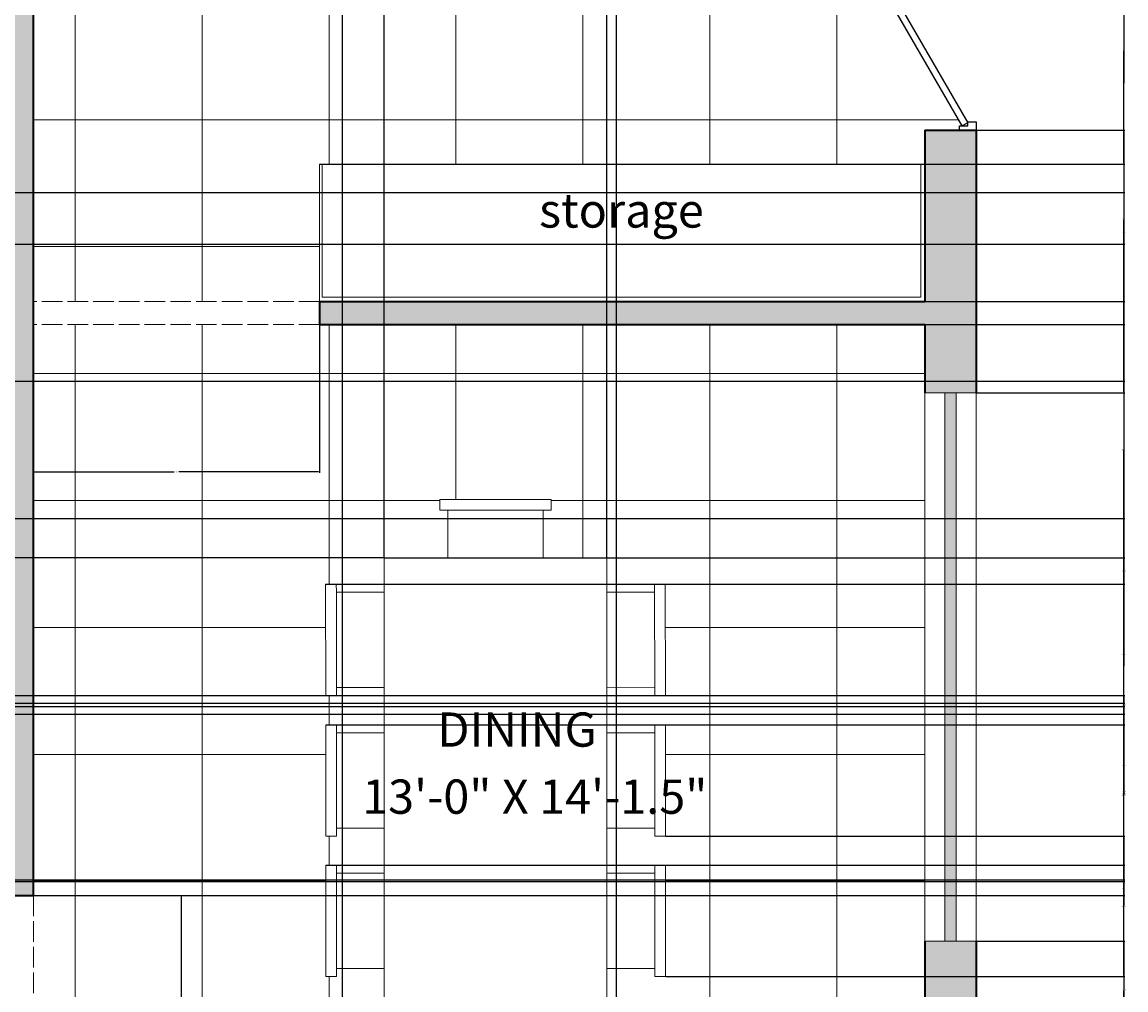
# Model space of a CAD drawing. Units: inches. Extents: x 6 to 575, y 34 to 566.
# Tile 16 of 21: x 382 to 575, y 262 to 432. Entities that reach past the tile are written whole.
import ezdxf

# ---------------------------------------------------------------- set-up
doc = ezdxf.new("R2010")
doc.units = ezdxf.units.IN
doc.linetypes.add('ACAD_ISO02W100', pattern=[15, 12, -3])
for name, color, linetype, lineweight in [('A-ANNO-DIMS', 2, 'Continuous', 18), ('A-ANNO-TEXT', 6, 'Continuous', 18), ('A-AREA-IDEN', 6, 'Continuous', 20), ('A-FLOR-CASE', 2, 'Continuous', 18), ('A-FLOR-PATT', 252, 'Continuous', 9), ('A-GLAZ-PATT', 4, 'Continuous', 9), ('A-WALL-OVHD', 7, 'ACAD_ISO02W100', 18), ('A-WALL-PATT', 251, 'Continuous', 9), ('DOORS', 3, 'Continuous', 25), ('FUR', 2, 'Continuous', 18), ('WALLS', 7, 'Continuous', 35), ('WINDOWS', 4, 'Continuous', 20)]:
    doc.layers.add(name, color=color, linetype=linetype, lineweight=lineweight)
doc.styles.add('PDF Arial Narrow', font='txt')
doc.styles.add('PDF Century Gothic', font='txt')
doc.styles.get("Standard").update_dxf_attribs({"font": 'arial.ttf'})
doc.dimstyles.get("Standard").update_dxf_attribs({"dimtxt": 0.18, "dimasz": 0.18, "dimexe": 0.18, "dimexo": 0.0625, "dimgap": 0.09, "dimtad": 0, "dimtih": 1, "dimtoh": 1, "dimdec": 4, "dimzin": 0, "dimdsep": 46, "dimtxsty": 'Standard', "dimcen": 0.09, "dimadec": 0, "dimazin": 0, "dimtfac": 1, "dimtdec": 4, "dimtofl": 0, "dimtmove": 0, "dimatfit": 3, "dimfxl": 1, "dimtolj": 1, "dimtzin": 0, "dimarcsym": 0})

# ---------------------------------------------------------------- blocks, each defined once
blk = doc.blocks.new('Door - Left Hung 36 in.')
blk.add_lwpolyline([(0.75, -1.3), (0, 0), (31.18, 18), (31.93, 16.7)], close=True)
blk.add_arc((0, 0), 36, 0, 37.3101)
blk = doc.blocks.new('CHAIR-DINING')
for points in [[(0, 1.4), (8.35, 1.4), (8.35, 0), (10.22, 0), (10.22, 19.51), (8.35, 19.51), (8.35, 18.1), (0, 18.1)], [(8.35, 18.1), (8.35, 1.4)]]:
    blk.add_lwpolyline(points)
blk = doc.blocks.new('*D44')
at = {"layer": 'A-ANNO-DIMS', "color": 0, "lineweight": -2, "transparency": 16777216}
for p, q in [((548.72, 270.8), (574.68, 270.8)), ((574.5, 270.62), (574.5, 237.48)), ((574.5, 203.98), (574.5, 237.12)), ((548.72, 203.8), (574.68, 203.8))]:
    blk.add_line(p, q, dxfattribs=at)
at = {"layer": 'A-ANNO-DIMS', "color": 0, "transparency": 16777216}
for points in [[(574.47, 270.62), (574.53, 270.62), (574.5, 270.8)], [(574.47, 203.98), (574.53, 203.98), (574.5, 203.8)]]:
    blk.add_solid(points, dxfattribs=at)
at = {"layer": 'Defpoints', "color": 0, "transparency": 16777216}
for p in [(548.66, 270.8), (574.5, 270.8), (548.66, 203.8)]:
    blk.add_point(p, dxfattribs=at)
at = {"layer": 'A-ANNO-DIMS', "color": 0, "transparency": 16777216, "insert": (574.5, 237.3), "char_height": 0.18, "attachment_point": 5}
blk.add_mtext('\\A1;67', dxfattribs=at)
blk = doc.blocks.new('*D45')
at = {"layer": 'A-ANNO-DIMS', "color": 0, "lineweight": -2, "transparency": 16777216}
for p, q in [((548.72, 366.8), (574.68, 366.8)), ((574.5, 366.62), (574.5, 318.98)), ((574.5, 270.98), (574.5, 318.62)), ((548.72, 270.8), (574.68, 270.8))]:
    blk.add_line(p, q, dxfattribs=at)
at = {"layer": 'A-ANNO-DIMS', "color": 0, "transparency": 16777216}
for points in [[(574.47, 366.62), (574.53, 366.62), (574.5, 366.8)], [(574.47, 270.98), (574.53, 270.98), (574.5, 270.8)]]:
    blk.add_solid(points, dxfattribs=at)
at = {"layer": 'Defpoints', "color": 0, "transparency": 16777216}
for p in [(548.66, 366.8), (574.5, 366.8), (548.66, 270.8)]:
    blk.add_point(p, dxfattribs=at)
at = {"layer": 'A-ANNO-DIMS', "color": 0, "transparency": 16777216, "insert": (574.5, 318.8), "char_height": 0.18, "attachment_point": 5}
blk.add_mtext('\\A1;96', dxfattribs=at)
blk = doc.blocks.new('*D46')
at = {"layer": 'A-ANNO-DIMS', "color": 0, "lineweight": -2, "transparency": 16777216}
for p, q in [((548.72, 412.8), (574.68, 412.8)), ((574.5, 412.62), (574.5, 389.98)), ((574.5, 366.98), (574.5, 389.62)), ((548.72, 366.8), (574.68, 366.8))]:
    blk.add_line(p, q, dxfattribs=at)
at = {"layer": 'A-ANNO-DIMS', "color": 0, "transparency": 16777216}
for points in [[(574.47, 412.62), (574.53, 412.62), (574.5, 412.8)], [(574.47, 366.98), (574.53, 366.98), (574.5, 366.8)]]:
    blk.add_solid(points, dxfattribs=at)
at = {"layer": 'Defpoints', "color": 0, "transparency": 16777216}
for p in [(548.66, 412.8), (574.5, 412.8), (548.66, 366.8)]:
    blk.add_point(p, dxfattribs=at)
at = {"layer": 'A-ANNO-DIMS', "color": 0, "transparency": 16777216, "insert": (574.5, 389.8), "char_height": 0.18, "attachment_point": 5}
blk.add_mtext('\\A1;46', dxfattribs=at)
blk = doc.blocks.new('*D47')
at = {"layer": 'A-ANNO-DIMS', "color": 0, "lineweight": -2, "transparency": 16777216}
for p, q in [((548.72, 440.8), (574.68, 440.8)), ((574.5, 440.62), (574.5, 426.98)), ((574.5, 412.98), (574.5, 426.62)), ((548.72, 412.8), (574.68, 412.8))]:
    blk.add_line(p, q, dxfattribs=at)
at = {"layer": 'A-ANNO-DIMS', "color": 0, "transparency": 16777216}
for points in [[(574.47, 440.62), (574.53, 440.62), (574.5, 440.8)], [(574.47, 412.98), (574.53, 412.98), (574.5, 412.8)]]:
    blk.add_solid(points, dxfattribs=at)
at = {"layer": 'Defpoints', "color": 0, "transparency": 16777216}
for p in [(548.66, 440.8), (574.5, 440.8), (548.66, 412.8)]:
    blk.add_point(p, dxfattribs=at)
at = {"layer": 'A-ANNO-DIMS', "color": 0, "transparency": 16777216, "insert": (574.5, 426.8), "char_height": 0.18, "attachment_point": 5}
blk.add_mtext('\\A1;28', dxfattribs=at)
blk = doc.blocks.new('*D51')
at = {"layer": 'A-ANNO-DIMS', "color": 0, "lineweight": -2, "transparency": 16777216}
for p, q in [((437.69, 435.25), (437.69, 33.76)), ((485.67, 435.25), (485.67, 33.76)), ((437.87, 33.94), (461.28, 33.94)), ((485.49, 33.94), (462.08, 33.94))]:
    blk.add_line(p, q, dxfattribs=at)
at = {"layer": 'A-ANNO-DIMS', "color": 0, "transparency": 16777216}
for points in [[(437.87, 33.97), (437.87, 33.91), (437.69, 33.94)], [(485.49, 33.97), (485.49, 33.91), (485.67, 33.94)]]:
    blk.add_solid(points, dxfattribs=at)
at = {"layer": 'Defpoints', "color": 0, "transparency": 16777216}
for p in [(437.69, 435.31), (485.67, 435.31), (485.67, 33.94)]:
    blk.add_point(p, dxfattribs=at)
at = {"layer": 'A-ANNO-DIMS', "color": 0, "transparency": 16777216, "insert": (461.68, 33.94), "char_height": 0.18, "attachment_point": 5}
blk.add_mtext('\\A1;47.98', dxfattribs=at)
blk = doc.blocks.new('*D53')
at = {"layer": 'A-ANNO-DIMS', "color": 0, "lineweight": -2, "transparency": 16777216}
for p, q in [((445.02, 338), (445.02, 565.81)), ((445.2, 565.63), (464.15, 565.63)), ((483.85, 565.63), (464.9, 565.63)), ((484.03, 338), (484.03, 565.81))]:
    blk.add_line(p, q, dxfattribs=at)
at = {"layer": 'A-ANNO-DIMS', "color": 0, "transparency": 16777216}
for points in [[(445.2, 565.66), (445.2, 565.6), (445.02, 565.63)], [(483.85, 565.66), (483.85, 565.6), (484.03, 565.63)]]:
    blk.add_solid(points, dxfattribs=at)
at = {"layer": 'Defpoints', "color": 0, "transparency": 16777216}
for p in [(484.03, 565.63), (445.02, 337.94), (484.03, 337.94)]:
    blk.add_point(p, dxfattribs=at)
at = {"layer": 'A-ANNO-DIMS', "color": 0, "transparency": 16777216, "insert": (464.53, 565.63), "char_height": 0.18, "attachment_point": 5}
blk.add_mtext('\\A1;39.01', dxfattribs=at)
blk = doc.blocks.new('*D54')
at = {"layer": 'A-ANNO-DIMS', "color": 0, "lineweight": -2, "transparency": 16777216}
for p, q in [((444.96, 337.94), (6.65, 337.94)), ((6.83, 337.76), (6.83, 299.11)), ((6.83, 260.1), (6.83, 298.75)), ((444.96, 259.92), (6.65, 259.92))]:
    blk.add_line(p, q, dxfattribs=at)
at = {"layer": 'A-ANNO-DIMS', "color": 0, "transparency": 16777216}
for points in [[(6.8, 337.76), (6.86, 337.76), (6.83, 337.94)], [(6.8, 260.1), (6.86, 260.1), (6.83, 259.92)]]:
    blk.add_solid(points, dxfattribs=at)
at = {"layer": 'Defpoints', "color": 0, "transparency": 16777216}
for p in [(6.83, 337.94), (445.02, 337.94), (445.02, 259.92)]:
    blk.add_point(p, dxfattribs=at)
at = {"layer": 'A-ANNO-DIMS', "color": 0, "transparency": 16777216, "insert": (6.83, 298.93), "char_height": 0.18, "attachment_point": 5}
blk.add_mtext('\\A1;78.02', dxfattribs=at)
blk = doc.blocks.new('*D57')
at = {"layer": 'A-ANNO-DIMS', "color": 0, "lineweight": -2, "transparency": 16777216}
for p, q in [((383.66, 378.74), (383.66, 352.79)), ((433.71, 378.74), (433.71, 352.79)), ((383.84, 352.97), (408.29, 352.97)), ((433.53, 352.97), (409.08, 352.97))]:
    blk.add_line(p, q, dxfattribs=at)
at = {"layer": 'A-ANNO-DIMS', "color": 0, "transparency": 16777216}
for points in [[(383.84, 353), (383.84, 352.94), (383.66, 352.97)], [(433.53, 353), (433.53, 352.94), (433.71, 352.97)]]:
    blk.add_solid(points, dxfattribs=at)
at = {"layer": 'Defpoints', "color": 0, "transparency": 16777216}
for p in [(383.66, 378.8), (433.71, 378.8), (383.66, 352.97)]:
    blk.add_point(p, dxfattribs=at)
at = {"layer": 'A-ANNO-DIMS', "color": 0, "transparency": 16777216, "insert": (408.68, 352.97), "char_height": 0.18, "attachment_point": 5}
blk.add_mtext('\\A1;50.05', dxfattribs=at)
blk = doc.blocks.new('*D58')
at = {"layer": 'A-ANNO-DIMS', "color": 0, "lineweight": -2, "transparency": 16777216}
for p, q in [((383.72, 278.8), (409.67, 278.8)), ((409.49, 278.62), (409.49, 251.98)), ((409.49, 224.98), (409.49, 251.62)), ((383.72, 224.8), (409.67, 224.8))]:
    blk.add_line(p, q, dxfattribs=at)
at = {"layer": 'A-ANNO-DIMS', "color": 0, "transparency": 16777216}
for points in [[(409.46, 278.62), (409.52, 278.62), (409.49, 278.8)], [(409.46, 224.98), (409.52, 224.98), (409.49, 224.8)]]:
    blk.add_solid(points, dxfattribs=at)
at = {"layer": 'Defpoints', "color": 0, "transparency": 16777216}
for p in [(383.66, 278.8), (383.66, 224.8), (409.49, 224.8)]:
    blk.add_point(p, dxfattribs=at)
at = {"layer": 'A-ANNO-DIMS', "color": 0, "transparency": 16777216, "insert": (409.49, 251.8), "char_height": 0.18, "attachment_point": 5}
blk.add_mtext('\\A1;54', dxfattribs=at)
blk = doc.blocks.new('*D65')
at = {"layer": 'A-ANNO-DIMS', "color": 0, "lineweight": -2, "transparency": 16777216}
for p, q in [((433.770494, 382.800984), (574.675816, 382.800984)), ((574.495816, 382.620984), (574.495816, 380.980984)), ((433.770494, 378.800984), (574.675816, 378.800984)), ((574.495816, 378.980984), (574.495816, 380.620984))]:
    blk.add_line(p, q, dxfattribs=at)
at = {"layer": 'A-ANNO-DIMS', "color": 0, "transparency": 16777216}
for points in [[(574.465816, 382.620984), (574.525816, 382.620984), (574.495816, 382.800984)], [(574.465816, 378.980984), (574.525816, 378.980984), (574.495816, 378.800984)]]:
    blk.add_solid(points, dxfattribs=at)
at = {"layer": 'Defpoints', "color": 0, "transparency": 16777216}
for p in [(433.707994, 382.800984), (574.495816, 382.800984), (433.707994, 378.800984)]:
    blk.add_point(p, dxfattribs=at)
at = {"layer": 'A-ANNO-DIMS', "color": 0, "transparency": 16777216, "insert": (574.495816, 380.800984), "char_height": 0.18, "attachment_point": 5}
blk.add_mtext('\\A1;4', dxfattribs=at)
blk = doc.blocks.new('*D120')
at = {"layer": 'A-ANNO-DIMS', "color": 0, "lineweight": -2, "transparency": 16777216}
for p, q in [((345.25, 401.87), (574.68, 401.87)), ((574.5, 401.69), (574.5, 357.07)), ((574.5, 312.09), (574.5, 356.71)), ((345.25, 311.91), (574.68, 311.91))]:
    blk.add_line(p, q, dxfattribs=at)
at = {"layer": 'A-ANNO-DIMS', "color": 0, "transparency": 16777216}
for points in [[(574.47, 401.69), (574.53, 401.69), (574.5, 401.87)], [(574.47, 312.09), (574.53, 312.09), (574.5, 311.91)]]:
    blk.add_solid(points, dxfattribs=at)
at = {"layer": 'Defpoints', "color": 0, "transparency": 16777216}
for p in [(345.19, 401.87), (574.5, 401.87), (345.19, 311.91)]:
    blk.add_point(p, dxfattribs=at)
at = {"layer": 'A-ANNO-DIMS', "color": 0, "transparency": 16777216, "insert": (574.5, 356.89), "char_height": 0.18, "attachment_point": 5}
blk.add_mtext('\\A1;89.96', dxfattribs=at)
blk = doc.blocks.new('*D121')
at = {"layer": 'A-ANNO-DIMS', "color": 0, "lineweight": -2, "transparency": 16777216}
for p, q in [((345.25, 311.91), (574.68, 311.91)), ((574.5, 311.73), (574.5, 296.75)), ((574.5, 281.42), (574.5, 296.39)), ((344.84, 281.24), (574.68, 281.24))]:
    blk.add_line(p, q, dxfattribs=at)
at = {"layer": 'A-ANNO-DIMS', "color": 0, "transparency": 16777216}
for points in [[(574.47, 311.73), (574.53, 311.73), (574.5, 311.91)], [(574.47, 281.42), (574.53, 281.42), (574.5, 281.24)]]:
    blk.add_solid(points, dxfattribs=at)
at = {"layer": 'Defpoints', "color": 0, "transparency": 16777216}
for p in [(345.19, 311.91), (574.5, 311.91), (344.78, 281.24)]:
    blk.add_point(p, dxfattribs=at)
at = {"layer": 'A-ANNO-DIMS', "color": 0, "transparency": 16777216, "insert": (574.5, 296.57), "char_height": 0.18, "attachment_point": 5}
blk.add_mtext('\\A1;30.673', dxfattribs=at)
blk = doc.blocks.new('*D123')
at = {"layer": 'A-ANNO-DIMS', "color": 0, "lineweight": -2, "transparency": 16777216}
for p, q in [((344.84, 281.24), (574.68, 281.24)), ((574.5, 281.06), (574.5, 280.2)), ((374.72, 278.8), (574.68, 278.8)), ((574.5, 278.98), (574.5, 279.84))]:
    blk.add_line(p, q, dxfattribs=at)
at = {"layer": 'A-ANNO-DIMS', "color": 0, "transparency": 16777216}
for points in [[(574.47, 281.06), (574.53, 281.06), (574.5, 281.24)], [(574.47, 278.98), (574.53, 278.98), (574.5, 278.8)]]:
    blk.add_solid(points, dxfattribs=at)
at = {"layer": 'Defpoints', "color": 0, "transparency": 16777216}
for p in [(344.78, 281.24), (574.5, 281.24), (374.66, 278.8)]:
    blk.add_point(p, dxfattribs=at)
at = {"layer": 'A-ANNO-DIMS', "color": 0, "transparency": 16777216, "insert": (574.5, 280.02), "char_height": 0.18, "attachment_point": 5}
blk.add_mtext('\\A1;2.435', dxfattribs=at)
blk = doc.blocks.new('*D124')
at = {"layer": 'A-ANNO-DIMS', "color": 0, "lineweight": -2, "transparency": 16777216}
for p, q in [((345.25, 401.87), (574.68, 401.87)), ((574.5, 401.69), (574.5, 397.53)), ((574.5, 393), (574.5, 397.16)), ((345.25, 392.82), (574.68, 392.82))]:
    blk.add_line(p, q, dxfattribs=at)
at = {"layer": 'A-ANNO-DIMS', "color": 0, "transparency": 16777216}
for points in [[(574.47, 401.69), (574.53, 401.69), (574.5, 401.87)], [(574.47, 393), (574.53, 393), (574.5, 392.82)]]:
    blk.add_solid(points, dxfattribs=at)
at = {"layer": 'Defpoints', "color": 0, "transparency": 16777216}
for p in [(345.19, 401.87), (574.5, 401.87), (345.19, 392.82)]:
    blk.add_point(p, dxfattribs=at)
at = {"layer": 'A-ANNO-DIMS', "color": 0, "transparency": 16777216, "insert": (574.5, 397.34), "char_height": 0.18, "attachment_point": 5}
blk.add_mtext('\\A1;9.05', dxfattribs=at)
blk = doc.blocks.new('*D125')
at = {"layer": 'A-ANNO-DIMS', "color": 0, "lineweight": -2, "transparency": 16777216}
for p, q in [((346.11, 368.87), (574.68, 368.87)), ((574.5, 368.69), (574.5, 357.03)), ((574.5, 345.01), (574.5, 356.67)), ((346.11, 344.83), (574.68, 344.83))]:
    blk.add_line(p, q, dxfattribs=at)
at = {"layer": 'A-ANNO-DIMS', "color": 0, "transparency": 16777216}
for points in [[(574.47, 368.69), (574.53, 368.69), (574.5, 368.87)], [(574.47, 345.01), (574.53, 345.01), (574.5, 344.83)]]:
    blk.add_solid(points, dxfattribs=at)
at = {"layer": 'Defpoints', "color": 0, "transparency": 16777216}
for p in [(346.05, 368.87), (574.5, 368.87), (346.05, 344.83)]:
    blk.add_point(p, dxfattribs=at)
at = {"layer": 'A-ANNO-DIMS', "color": 0, "transparency": 16777216, "insert": (574.5, 356.85), "char_height": 0.18, "attachment_point": 5}
blk.add_mtext('\\A1;24.03', dxfattribs=at)
blk = doc.blocks.new('*D128')
at = {"layer": 'A-ANNO-DIMS', "color": 0, "lineweight": -2, "transparency": 16777216}
for p, q in [((288.92, 312.45), (574.68, 312.45)), ((574.5, 312.27), (574.5, 297.18)), ((574.5, 281.73), (574.5, 296.82)), ((293.5, 281.55), (574.68, 281.55))]:
    blk.add_line(p, q, dxfattribs=at)
at = {"layer": 'A-ANNO-DIMS', "color": 0, "transparency": 16777216}
for points in [[(574.47, 312.27), (574.53, 312.27), (574.5, 312.45)], [(574.47, 281.73), (574.53, 281.73), (574.5, 281.55)]]:
    blk.add_solid(points, dxfattribs=at)
at = {"layer": 'Defpoints', "color": 0, "transparency": 16777216}
for p in [(288.86, 312.45), (574.5, 312.45), (293.44, 281.55)]:
    blk.add_point(p, dxfattribs=at)
at = {"layer": 'A-ANNO-DIMS', "color": 0, "transparency": 16777216, "insert": (574.5, 297), "char_height": 0.18, "attachment_point": 5}
blk.add_mtext('\\A1;30.91', dxfattribs=at)
blk = doc.blocks.new('*D130')
at = {"layer": 'A-ANNO-DIMS', "color": 0, "lineweight": -2, "transparency": 16777216}
for p, q in [((343.34, 313.82), (574.68, 313.82)), ((574.5, 313.64), (574.5, 312.36)), ((574.5, 310.72), (574.5, 312)), ((330.47, 310.54), (574.68, 310.54))]:
    blk.add_line(p, q, dxfattribs=at)
at = {"layer": 'A-ANNO-DIMS', "color": 0, "transparency": 16777216}
for points in [[(574.47, 313.64), (574.53, 313.64), (574.5, 313.82)], [(574.47, 310.72), (574.53, 310.72), (574.5, 310.54)]]:
    blk.add_solid(points, dxfattribs=at)
at = {"layer": 'Defpoints', "color": 0, "transparency": 16777216}
for p in [(343.28, 313.82), (574.5, 313.82), (330.4, 310.54)]:
    blk.add_point(p, dxfattribs=at)
at = {"layer": 'A-ANNO-DIMS', "color": 0, "transparency": 16777216, "insert": (574.5, 312.18), "char_height": 0.18, "attachment_point": 5}
blk.add_mtext('\\A1;3.277', dxfattribs=at)
blk = doc.blocks.new('*D140')
at = {"layer": 'A-ANNO-DIMS', "color": 0, "lineweight": -2, "transparency": 16777216}
for p, q in [((445.08, 337.94), (574.68, 337.94)), ((574.5, 337.76), (574.5, 335.81)), ((574.5, 333.49), (574.5, 335.44)), ((434.85, 333.31), (574.68, 333.31))]:
    blk.add_line(p, q, dxfattribs=at)
at = {"layer": 'A-ANNO-DIMS', "color": 0, "transparency": 16777216}
for points in [[(574.47, 337.76), (574.53, 337.76), (574.5, 337.94)], [(574.47, 333.49), (574.53, 333.49), (574.5, 333.31)]]:
    blk.add_solid(points, dxfattribs=at)
at = {"layer": 'Defpoints', "color": 0, "transparency": 16777216}
for p in [(445.02, 337.94), (434.79, 333.31), (574.5, 333.31)]:
    blk.add_point(p, dxfattribs=at)
at = {"layer": 'A-ANNO-DIMS', "color": 0, "transparency": 16777216, "insert": (574.5, 335.62), "char_height": 0.18, "attachment_point": 5}
blk.add_mtext('\\A1;4.631', dxfattribs=at)
blk = doc.blocks.new('*D141')
at = {"layer": 'A-ANNO-DIMS', "color": 0, "lineweight": -2, "transparency": 16777216}
for p, q in [((434.85, 333.31), (574.68, 333.31)), ((574.5, 333.13), (574.5, 321.18)), ((574.5, 308.86), (574.5, 320.81)), ((434.86, 308.68), (574.68, 308.68))]:
    blk.add_line(p, q, dxfattribs=at)
at = {"layer": 'A-ANNO-DIMS', "color": 0, "transparency": 16777216}
for points in [[(574.47, 333.13), (574.53, 333.13), (574.5, 333.31)], [(574.47, 308.86), (574.53, 308.86), (574.5, 308.68)]]:
    blk.add_solid(points, dxfattribs=at)
at = {"layer": 'Defpoints', "color": 0, "transparency": 16777216}
for p in [(434.79, 333.31), (434.8, 308.68), (574.5, 308.68)]:
    blk.add_point(p, dxfattribs=at)
at = {"layer": 'A-ANNO-DIMS', "color": 0, "transparency": 16777216, "insert": (574.5, 321), "char_height": 0.18, "attachment_point": 5}
blk.add_mtext('\\A1;24.626', dxfattribs=at)
blk = doc.blocks.new('*D142')
at = {"layer": 'A-ANNO-DIMS', "color": 0, "lineweight": -2, "transparency": 16777216}
for p, q in [((434.86, 308.68), (574.68, 308.68)), ((574.5, 308.5), (574.5, 296.58)), ((574.5, 284.29), (574.5, 296.21)), ((434.86, 284.11), (574.68, 284.11))]:
    blk.add_line(p, q, dxfattribs=at)
at = {"layer": 'A-ANNO-DIMS', "color": 0, "transparency": 16777216}
for points in [[(574.47, 308.5), (574.53, 308.5), (574.5, 308.68)], [(574.47, 284.29), (574.53, 284.29), (574.5, 284.11)]]:
    blk.add_solid(points, dxfattribs=at)
at = {"layer": 'Defpoints', "color": 0, "transparency": 16777216}
for p in [(434.8, 308.68), (434.8, 284.11), (574.5, 284.11)]:
    blk.add_point(p, dxfattribs=at)
at = {"layer": 'A-ANNO-DIMS', "color": 0, "transparency": 16777216, "insert": (574.5, 296.39), "char_height": 0.18, "attachment_point": 5}
blk.add_mtext('\\A1;24.576', dxfattribs=at)
blk = doc.blocks.new('*D146')
at = {"layer": 'A-ANNO-DIMS', "color": 0, "lineweight": -2, "transparency": 16777216}
for p, q in [((494.31, 289.18), (574.68, 289.18)), ((574.5, 289), (574.5, 277.07)), ((574.5, 264.78), (574.5, 276.71)), ((494.31, 264.6), (574.68, 264.6))]:
    blk.add_line(p, q, dxfattribs=at)
at = {"layer": 'A-ANNO-DIMS', "color": 0, "transparency": 16777216}
for points in [[(574.47, 289), (574.53, 289), (574.5, 289.18)], [(574.47, 264.78), (574.53, 264.78), (574.5, 264.6)]]:
    blk.add_solid(points, dxfattribs=at)
at = {"layer": 'Defpoints', "color": 0, "transparency": 16777216}
for p in [(494.25, 289.18), (574.5, 289.18), (494.25, 264.6)]:
    blk.add_point(p, dxfattribs=at)
at = {"layer": 'A-ANNO-DIMS', "color": 0, "transparency": 16777216, "insert": (574.5, 276.89), "char_height": 0.18, "attachment_point": 5}
blk.add_mtext('\\A1;24.576', dxfattribs=at)
blk = doc.blocks.new('*D147')
at = {"layer": 'A-ANNO-DIMS', "color": 0, "lineweight": -2, "transparency": 16777216}
for p, q in [((494.35, 313.82), (574.68, 313.82)), ((574.5, 313.64), (574.5, 301.68)), ((574.5, 289.36), (574.5, 301.32)), ((494.31, 289.18), (574.68, 289.18))]:
    blk.add_line(p, q, dxfattribs=at)
at = {"layer": 'A-ANNO-DIMS', "color": 0, "transparency": 16777216}
for points in [[(574.47, 313.64), (574.53, 313.64), (574.5, 313.82)], [(574.47, 289.36), (574.53, 289.36), (574.5, 289.18)]]:
    blk.add_solid(points, dxfattribs=at)
at = {"layer": 'Defpoints', "color": 0, "transparency": 16777216}
for p in [(494.28, 313.82), (574.5, 313.82), (494.25, 289.18)]:
    blk.add_point(p, dxfattribs=at)
at = {"layer": 'A-ANNO-DIMS', "color": 0, "transparency": 16777216, "insert": (574.5, 301.5), "char_height": 0.18, "attachment_point": 5}
blk.add_mtext('\\A1;24.64', dxfattribs=at)
blk = doc.blocks.new('*D148')
at = {"layer": 'A-ANNO-DIMS', "color": 0, "lineweight": -2, "transparency": 16777216}
for p, q in [((494.31, 264.6), (574.68, 264.6)), ((574.5, 264.42), (574.5, 262.44)), ((574.5, 260.1), (574.5, 262.08)), ((484.09, 259.92), (574.68, 259.92))]:
    blk.add_line(p, q, dxfattribs=at)
at = {"layer": 'A-ANNO-DIMS', "color": 0, "transparency": 16777216}
for points in [[(574.47, 264.42), (574.53, 264.42), (574.5, 264.6)], [(574.47, 260.1), (574.53, 260.1), (574.5, 259.92)]]:
    blk.add_solid(points, dxfattribs=at)
at = {"layer": 'Defpoints', "color": 0, "transparency": 16777216}
for p in [(494.25, 264.6), (574.5, 264.6), (484.03, 259.92)]:
    blk.add_point(p, dxfattribs=at)
at = {"layer": 'A-ANNO-DIMS', "color": 0, "transparency": 16777216, "insert": (574.5, 262.26), "char_height": 0.18, "attachment_point": 5}
blk.add_mtext('\\A1;4.681', dxfattribs=at)
blk = doc.blocks.new('*D151')
at = {"layer": 'A-ANNO-DIMS', "color": 0, "lineweight": -2, "transparency": 16777216}
for p, q in [((437.75, 435.31), (574.68, 435.31)), ((574.5, 435.13), (574.5, 421.25)), ((574.5, 407.01), (574.5, 420.89)), ((433.77, 406.83), (574.68, 406.83))]:
    blk.add_line(p, q, dxfattribs=at)
at = {"layer": 'A-ANNO-DIMS', "color": 0, "transparency": 16777216}
for points in [[(574.47, 435.13), (574.53, 435.13), (574.5, 435.31)], [(574.47, 407.01), (574.53, 407.01), (574.5, 406.83)]]:
    blk.add_solid(points, dxfattribs=at)
at = {"layer": 'Defpoints', "color": 0, "transparency": 16777216}
for p in [(437.69, 435.31), (433.71, 406.83), (574.5, 406.83)]:
    blk.add_point(p, dxfattribs=at)
at = {"layer": 'A-ANNO-DIMS', "color": 0, "transparency": 16777216, "insert": (574.5, 421.07), "char_height": 0.18, "attachment_point": 5}
blk.add_mtext('\\A1;28.48', dxfattribs=at)
blk = doc.blocks.new('*D154')
at = {"layer": 'A-ANNO-DIMS', "color": 0, "lineweight": -2, "transparency": 16777216}
for p, q in [((433.77, 406.83), (574.68, 406.83)), ((574.5, 406.65), (574.5, 395)), ((574.5, 382.98), (574.5, 394.63)), ((433.77, 382.8), (574.68, 382.8))]:
    blk.add_line(p, q, dxfattribs=at)
at = {"layer": 'A-ANNO-DIMS', "color": 0, "transparency": 16777216}
for points in [[(574.47, 406.65), (574.53, 406.65), (574.5, 406.83)], [(574.47, 382.98), (574.53, 382.98), (574.5, 382.8)]]:
    blk.add_solid(points, dxfattribs=at)
at = {"layer": 'Defpoints', "color": 0, "transparency": 16777216}
for p in [(433.71, 406.83), (574.5, 406.83), (433.71, 382.8)]:
    blk.add_point(p, dxfattribs=at)
at = {"layer": 'A-ANNO-DIMS', "color": 0, "transparency": 16777216, "insert": (574.5, 394.82), "char_height": 0.18, "attachment_point": 5}
blk.add_mtext('\\A1;24.03', dxfattribs=at)

msp = doc.modelspace()

# ---------------------------------------------------------------- hatches: boundary and pattern name
at = {"layer": 'A-FLOR-PATT'}
h = msp.add_hatch(dxfattribs=at)
h.set_pattern_fill('NET', color=256, scale=7)
h.set_pattern_definition([(0, (-98.035, 170.147), (0, 22.225), []), (90, (-98.035, 170.147), (-22.225, 1e-15), [])])
h.paths.add_polyline_path([(539.6586, 366.801), (539.6586, 378.801), (433.708, 378.801), (383.6586, 378.801), (383.6586, 278.801), (383.6586, 224.801), (383.6586, 212.801), (407.6586, 212.801), (515.6586, 212.801), (539.6586, 212.801), (539.6586, 270.801)])
h.paths.add_polyline_path([(434.8003, 333.3365), (436.6727, 333.3365), (436.6727, 331.9322), (445.0208, 331.9322), (445.0208, 337.9397), (456.1776, 337.9397), (456.1776, 346.2878), (454.7733, 346.2878), (454.7733, 348.1603), (474.2782, 348.1603), (474.2782, 346.2878), (472.8738, 346.2878), (472.8738, 337.9397), (484.0307, 337.9397), (484.0307, 331.9322), (492.3788, 331.9322), (492.3788, 333.3365), (494.2512, 333.3365), (494.2512, 313.8316), (492.3788, 313.8316), (492.3788, 315.158), (484.0307, 315.158), (484.0307, 307.278), (492.3788, 307.278), (492.3788, 308.6823), (494.2512, 308.6823), (494.2512, 289.1774), (492.3788, 289.1774), (492.3788, 290.5818), (484.0307, 290.5818), (484.0307, 282.7018), (492.3788, 282.7018), (492.3788, 284.1062), (494.2512, 284.1062), (494.2512, 264.6013), (492.3788, 264.6013), (492.3788, 266.0056), (484.0307, 266.0056), (484.0307, 259.9201), (472.8738, 259.9201), (472.8738, 251.572), (474.2782, 251.572), (474.2782, 249.6995), (454.7733, 249.6995), (454.7733, 251.572), (456.1776, 251.572), (456.1776, 259.9201), (445.0208, 259.9201), (445.0208, 266.0056), (436.6727, 266.0056), (436.6727, 264.6013), (434.8003, 264.6013), (434.8003, 284.1062), (436.6727, 284.1062), (436.6727, 282.7018), (445.0208, 282.7018), (445.0208, 290.5818), (436.6727, 290.5818), (436.6727, 289.1774), (434.8003, 289.1774), (434.8003, 308.6823), (436.6727, 308.6823), (436.6727, 307.278), (445.0208, 307.278), (445.0208, 315.158), (436.6727, 315.158), (436.6727, 313.8316), (434.8003, 313.8316)], flags=16)
h.paths.add_polyline_path([(532.9619, 436.5144), (533.9192, 437.0672), (533.9307, 437.0472, -0.12106636), (546.2274, 440.0689), (539.6586, 440.801), (539.6586, 450.6781), (515.7066, 450.6781), (515.7066, 507.3203), (407.6494, 507.3203), (407.6494, 449.3517), (383.6586, 449.3517), (383.6586, 382.801), (433.708, 382.801), (433.708, 406.831), (539.6586, 406.831), (539.6586, 412.801), (545.7108, 412.801), (545.7108, 414.4327)])
h.paths.add_polyline_path([(437.687, 435.3082), (437.687, 471.3533), (485.6691, 471.3533), (485.6691, 435.3082)], flags=16)
at = {"layer": 'A-GLAZ-PATT'}
h = msp.add_hatch(color=256, dxfattribs=at)
h.dxf.hatch_style = 1
h.paths.add_polyline_path([(36.1586, 224.801), (38.1586, 224.801), (38.1586, 272.801), (36.1586, 272.801)])
h.paths.add_polyline_path([(167.6586, 207.301), (167.6586, 209.301), (71.6586, 209.301), (71.6586, 207.301)])
h.paths.add_polyline_path([(264.6586, 219.301), (264.6586, 221.301), (246.6586, 221.301), (246.6586, 219.301)])
h.paths.add_polyline_path([(316.6586, 221.301), (316.6586, 219.301), (334.6586, 219.301), (334.6586, 221.301)])
h.paths.add_polyline_path([(515.6586, 207.301), (515.6586, 209.301), (407.6586, 209.301), (407.6586, 207.301)])
h.paths.add_polyline_path([(543.1586, 270.801), (545.1586, 270.801), (545.1586, 366.801), (543.1586, 366.801)])
h.paths.add_polyline_path([(407.9436, 536.301), (407.9436, 534.301), (455.9436, 534.301), (455.9436, 536.301)])
h.paths.add_polyline_path([(272.6586, 536.301), (272.6586, 534.301), (320.6586, 534.301), (320.6586, 536.301)])
at = {"layer": 'A-WALL-PATT'}
h = msp.add_hatch(color=256, dxfattribs=at)
h.dxf.hatch_style = 1
h.paths.add_polyline_path([(160.6586, 539.801), (32.6586, 539.801), (32.6586, 272.801), (41.6586, 272.801), (41.6586, 286.0643), (41.6586, 358.0764), (41.6586, 379.0637), (41.6586, 407.7709), (41.6194, 407.7709), (41.6194, 431.801), (82.8918, 431.801), (82.8918, 440.801), (65.6494, 440.801), (65.6494, 440.7732), (41.6194, 440.7732), (41.6194, 515.5941), (41.6586, 530.801), (117.6586, 530.801), (117.6586, 474.801), (120.6068, 474.801), (121.6586, 474.801), (121.6586, 530.801), (137.4275, 530.801), (137.4275, 530.8356), (141.2505, 530.8356), (160.6586, 530.801)])
h.paths.add_polyline_path([(71.6586, 212.801), (41.6586, 212.801), (41.6586, 224.801), (32.6586, 224.801), (32.6586, 203.801), (71.6586, 203.801)])
h.paths.add_polyline_path([(206.6586, 215.801), (246.6586, 215.801), (246.6586, 224.801), (206.6586, 224.801), (206.6586, 230.801), (201.8157, 230.801), (197.6586, 230.801), (197.6586, 212.801), (167.6586, 212.801), (167.6586, 203.801), (206.6586, 203.801)])
h.paths.add_polyline_path([(383.6586, 224.801), (334.6586, 224.801), (334.6586, 215.801), (374.6586, 215.801), (374.6586, 203.801), (384.0753, 203.801), (407.6586, 203.801), (407.6586, 212.801), (383.6586, 212.801)])
h.paths.add_polyline_path([(548.6586, 270.801), (539.6586, 270.801), (539.6586, 212.801), (515.6586, 212.801), (515.6586, 203.801), (548.6586, 203.801)])
h.paths.add_polyline_path([(548.6586, 412.801), (545.7108, 412.801), (539.6586, 412.801), (539.6586, 382.801), (433.708, 382.801), (433.708, 378.801), (539.6586, 378.801), (539.6586, 366.801), (548.6586, 366.801)])
h.paths.add_polyline_path([(548.6586, 539.801), (455.9436, 539.801), (455.9436, 530.801), (539.6586, 530.801), (539.6586, 440.801), (548.6586, 440.801)])
h.paths.add_polyline_path([(407.9436, 539.801), (362.6586, 539.801), (362.6586, 530.801), (374.6586, 530.801), (374.6586, 452.801), (354.6586, 452.801), (354.6586, 448.801), (374.6586, 448.801), (374.6586, 278.801), (383.6586, 278.801), (383.6586, 530.801), (407.9436, 530.801)])
h.paths.add_polyline_path([(338.6586, 539.801), (320.6586, 539.801), (320.6586, 530.801), (322.6586, 530.801), (322.6586, 448.801), (326.6586, 448.801), (326.6586, 530.801), (338.6586, 530.801)])
h.paths.add_polyline_path([(272.6586, 539.801), (184.6586, 539.801), (184.6586, 530.801), (197.6586, 530.801), (197.6586, 440.801), (176.6714, 440.801), (121.6586, 440.801), (121.6586, 446.801), (117.6586, 446.801), (117.6586, 440.801), (111.6586, 440.801), (111.6586, 431.801), (197.6586, 431.801), (197.6586, 407.7709), (197.6586, 276.801), (206.6586, 276.801), (206.6586, 530.801), (272.6586, 530.801)])

# ---------------------------------------------------------------- linework, layer by layer
at = {"layer": 'A-FLOR-CASE'}
for points in [[(433.708, 406.831), (539.6586, 406.831), (539.6586, 382.801), (433.708, 382.801)], [(434.1761, 406.831), (538.9565, 406.831), (538.9565, 383.5812), (434.1761, 383.5812)]]:
    msp.add_lwpolyline(points, close=True, dxfattribs=at)
at = {"layer": 'A-WALL-OVHD', "ltscale": 0.3}
for p, q in [((433.708, 382.801), (383.6586, 382.801)), ((433.708, 378.801), (383.6586, 378.801)), ((383.6586, 278.801), (383.6586, 224.801))]:
    msp.add_line(p, q, dxfattribs=at)
at = {"layer": 'DOORS'}
msp.add_lwpolyline([(548.6586, 414.2749), (548.6586, 412.801), (545.7108, 412.801), (545.7108, 413.538), (547.1847, 413.538), (547.1847, 414.2749)], close=True, dxfattribs=at)
at = {"layer": 'FUR'}
msp.add_lwpolyline([(484.0307, 337.9397), (484.0307, 259.9201), (445.0208, 259.9201), (445.0208, 337.9397)], close=True, dxfattribs=at)
at = {"layer": 'WALLS'}
for p, q in [((383.6586, 278.801), (383.6586, 530.801)), ((539.6586, 412.801), (548.6586, 412.801)), ((539.6586, 412.801), (539.6586, 382.801)), ((548.6586, 412.801), (548.6586, 366.801)), ((433.708, 382.801), (539.6586, 382.801)), ((433.708, 382.801), (433.708, 378.801)), ((433.708, 378.801), (539.6586, 378.801)), ((539.6586, 378.801), (539.6586, 366.801)), ((374.6586, 278.801), (383.6586, 278.801)), ((539.6586, 270.801), (539.6586, 212.801)), ((548.6586, 270.801), (548.6586, 203.801))]:
    msp.add_line(p, q, dxfattribs=at)
at = {"layer": 'WINDOWS'}
for p, q in [((539.6586, 366.801), (548.6586, 366.801)), ((548.6586, 366.801), (539.6586, 366.801)), ((543.1586, 270.801), (543.1586, 366.801)), ((545.1586, 270.801), (545.1586, 366.801)), ((539.6586, 270.801), (548.6586, 270.801)), ((548.6586, 270.801), (539.6586, 270.801))]:
    msp.add_line(p, q, dxfattribs=at)
msp.add_lwpolyline([(539.6586, 270.801), (548.6586, 270.801), (548.6586, 366.801), (539.6586, 366.801)], close=True, dxfattribs=at)

# ---------------------------------------------------------------- block references
at = {"layer": 'DOORS', "xscale": 0.7369707940286819, "yscale": 0.7369707940286819, "zscale": 0.7369707940286819, "rotation": 90.00000000000003}
msp.add_blockref('Door - Left Hung 36 in.', (546.2274, 413.538), dxfattribs=at)
at = {"layer": 'FUR'}
for p, rotation in [((474.2786, 337.94), 90.0000000000009), ((445.007, 333.3233), 180.0790637560415), ((484.0624, 313.7852), 0.1840806969806376), ((445.0205, 308.6828), 180), ((445.0205, 284.1066), 180)]:
    msp.add_blockref('CHAIR-DINING', p, dxfattribs=dict(at, rotation=rotation))
for p in [(484.031, 289.177), (484.031, 264.6008)]:
    msp.add_blockref('CHAIR-DINING', p, dxfattribs=at)

# ---------------------------------------------------------------- texts
at = {"layer": 'A-ANNO-TEXT', "insert": (472.1556, 397.9638), "char_height": 6.00051, "attachment_point": 4, "style": 'PDF Century Gothic'}
msp.add_mtext('storage', dxfattribs=at)
at = {"layer": 'A-AREA-IDEN', "attachment_point": 4, "style": 'PDF Arial Narrow'}
for s, insert, char_height in [('DINING', (454.3398, 307.0684), 6.0005), ('13\'-0" X 14\'-1.5"', (441.1832, 295.3274), 6.000503)]:
    msp.add_mtext(s, dxfattribs=dict(at, insert=insert, char_height=char_height))

# ---------------------------------------------------------------- dimensions: what is measured, and where the dimension line sits
at = {"layer": 'A-ANNO-DIMS'}
for base, p1, p2, picture, middle in [((484.0307, 565.631), (445.0208, 337.9397), (484.0307, 337.9397), '*D53', (464.5257, 565.631)), ((485.6691, 33.9447), (437.687, 435.3082), (485.6691, 435.3082), '*D51', (461.678, 33.9447))]:
    dim = msp.add_linear_dim(base=base, p1=p1, p2=p2, dimstyle='Standard', override={"dimdec": 2, "dimlfac": 1, "dimrnd": 0, "dimzin": 0, "dimdsep": 46, "dimlunit": 2}, dxfattribs=at)
    dim.commit()
    dim.dimension.update_dxf_attribs({"geometry": picture, "text_midpoint": middle})
for base, p1, p2, angle, override, picture, middle in [((574.4958, 440.801), (548.6586, 412.801), (548.6586, 440.801), 90, {"dimdec": 0, "dimlfac": 1, "dimrnd": 0, "dimzin": 0, "dimdsep": 46, "dimlunit": 2}, '*D47', (574.4958, 426.801)), ((574.4958, 406.831), (437.687, 435.3082), (433.708, 406.831), 90, {"dimdec": 2, "dimlfac": 1, "dimrnd": 0, "dimzin": 0, "dimdsep": 46, "dimlunit": 2}, '*D151', (574.4958, 421.0696)), ((574.4958, 412.801), (548.6586, 366.801), (548.6586, 412.801), 90, {"dimdec": 0, "dimlfac": 1, "dimrnd": 0, "dimzin": 0, "dimdsep": 46, "dimlunit": 2}, '*D46', (574.4958, 389.801)), ((574.4958, 406.831), (433.708, 382.801), (433.708, 406.831), 90, {"dimdec": 2, "dimlfac": 1, "dimrnd": 0, "dimzin": 0, "dimdsep": 46, "dimlunit": 2}, '*D154', (574.4958, 394.816)), ((574.4958, 401.8691), (345.1899, 311.909), (345.1899, 401.8691), 90, {"dimdec": 2, "dimlfac": 1, "dimrnd": 0, "dimzin": 0, "dimdsep": 46, "dimlunit": 2}, '*D120', (574.4958, 356.889)), ((574.4958, 401.8691), (345.1899, 392.8186), (345.1899, 401.8691), 90, {"dimdec": 2, "dimlfac": 1, "dimrnd": 0, "dimzin": 0, "dimdsep": 46, "dimlunit": 2}, '*D124', (574.4958, 397.3439)), ((574.4958, 382.801), (433.708, 378.801), (433.708, 382.801), 90, {"dimdec": 0, "dimlfac": 1, "dimrnd": 0, "dimzin": 0, "dimdsep": 46, "dimlunit": 2}, '*D65', (574.4958, 380.801)), ((383.6586, 352.971), (433.708, 378.801), (383.6586, 378.801), 180, {"dimdec": 2, "dimlfac": 1, "dimrnd": 0, "dimzin": 0, "dimdsep": 46, "dimlunit": 2}, '*D57', (408.6833, 352.971)), ((574.4958, 368.8656), (346.0482, 344.8346), (346.0482, 368.8656), 90, {"dimdec": 2, "dimlfac": 1, "dimrnd": 0, "dimzin": 0, "dimdsep": 46, "dimlunit": 2}, '*D125', (574.4958, 356.8501)), ((574.4958, 366.801), (548.6586, 270.801), (548.6586, 366.801), 90, {"dimdec": 0, "dimlfac": 1, "dimrnd": 0, "dimzin": 0, "dimdsep": 46, "dimlunit": 2}, '*D45', (574.4958, 318.801)), ((6.8286, 337.9397), (445.0208, 259.9201), (445.0208, 337.9397), 90, {"dimdec": 2, "dimlfac": 1, "dimrnd": 0, "dimzin": 0, "dimdsep": 46, "dimlunit": 2}, '*D54', (6.8286, 298.9299)), ((574.4958, 333.3088), (445.0208, 337.9397), (434.7868, 333.3088), 90, {"dimdec": 3, "dimlfac": 1, "dimrnd": 0, "dimzin": 0, "dimdsep": 46, "dimlunit": 2}, '*D140', (574.4958, 335.6242)), ((574.49582, 308.68234), (434.78681, 333.30876), (434.80027, 308.68234), 90, {"dimdec": 3, "dimlfac": 1, "dimrnd": 0, "dimzin": 0, "dimdsep": 46, "dimlunit": 2}, '*D141', (574.49582, 320.99555)), ((574.4958, 313.8205), (330.4045, 310.5435), (343.2784, 313.8205), 90, {"dimdec": 3, "dimlfac": 1, "dimrnd": 0, "dimzin": 0, "dimdsep": 46, "dimlunit": 2}, '*D130', (574.4958, 312.182)), ((574.4958, 313.8185), (494.2512, 289.1774), (494.2825, 313.8185), 90, {"dimdec": 2, "dimlfac": 1, "dimrnd": 0, "dimzin": 0, "dimdsep": 46, "dimlunit": 2}, '*D147', (574.4958, 301.4979)), ((574.4958, 312.455), (293.4402, 281.5479), (288.8575, 312.455), 90, {"dimdec": 2, "dimlfac": 1, "dimrnd": 0, "dimzin": 0, "dimdsep": 46, "dimlunit": 2}, '*D128', (574.4958, 297.0014)), ((574.4958, 311.909), (344.7771, 281.2358), (345.1899, 311.909), 90, {"dimdec": 3, "dimlfac": 1, "dimrnd": 0, "dimzin": 0, "dimdsep": 46, "dimlunit": 2}, '*D121', (574.4958, 296.5724)), ((574.4958, 284.1062), (434.8003, 308.6823), (434.8003, 284.1062), 90, {"dimdec": 3, "dimlfac": 1, "dimrnd": 0, "dimzin": 0, "dimdsep": 46, "dimlunit": 2}, '*D142', (574.4958, 296.3942)), ((574.4958, 289.1774), (494.2512, 264.6013), (494.2512, 289.1774), 90, {"dimdec": 3, "dimlfac": 1, "dimrnd": 0, "dimzin": 0, "dimdsep": 46, "dimlunit": 2}, '*D146', (574.4958, 276.8893)), ((574.4958, 281.2358), (374.6586, 278.801), (344.7771, 281.2358), 90, {"dimdec": 3, "dimlfac": 1, "dimrnd": 0, "dimzin": 0, "dimdsep": 46, "dimlunit": 2}, '*D123', (574.4958, 280.0184)), ((409.4886, 224.801), (383.6586, 278.801), (383.6586, 224.801), 270, {"dimdec": 0, "dimlfac": 1, "dimrnd": 0, "dimzin": 0, "dimdsep": 46, "dimlunit": 2}, '*D58', (409.4886, 251.801)), ((574.4958, 270.801), (548.6586, 203.801), (548.6586, 270.801), 90, {"dimdec": 0, "dimlfac": 1, "dimrnd": 0, "dimzin": 0, "dimdsep": 46, "dimlunit": 2}, '*D44', (574.4958, 237.301)), ((574.4958, 264.6013), (484.0307, 259.9201), (494.2512, 264.6013), 90, {"dimdec": 3, "dimlfac": 1, "dimrnd": 0, "dimzin": 0, "dimdsep": 46, "dimlunit": 2}, '*D148', (574.4958, 262.2607))]:
    dim = msp.add_linear_dim(base=base, p1=p1, p2=p2, angle=angle, dimstyle='Standard', override=override, dxfattribs=at)
    dim.commit()
    dim.dimension.update_dxf_attribs({"geometry": picture, "text_midpoint": middle})

doc.saveas('drawing.dxf')
